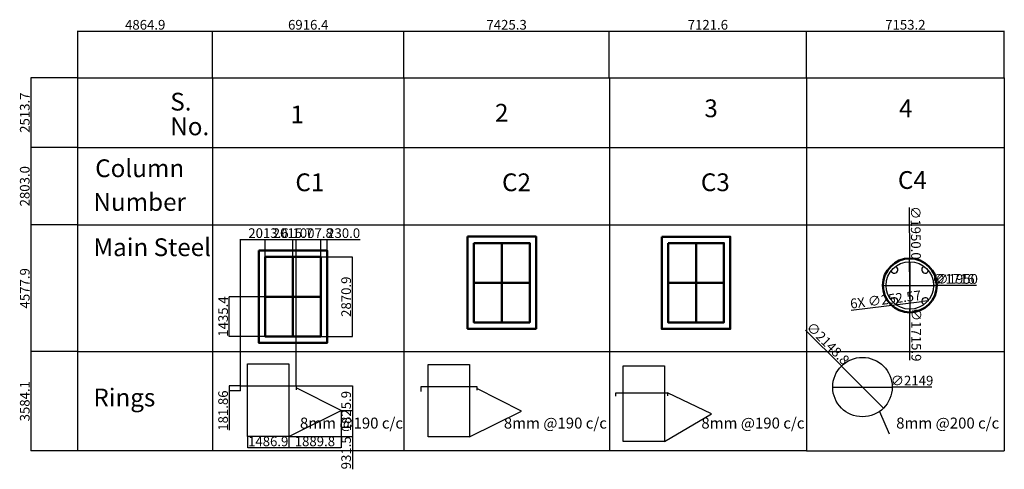
# Model space of a CAD drawing. Units: millimetres. Extents: x -2405 to 73447, y 417 to 55353.
# Tile 1 of 3: x 1710 to 37295, y 417 to 16669. Entities that reach past the tile are written whole.
import ezdxf

# ---------------------------------------------------------------- set-up
doc = ezdxf.new("R2010")
doc.units = ezdxf.units.MM
for name, color, linetype, lineweight in [('S-ANNO-DIMS', 2, 'Continuous', 18), ('S-ANNO-SCHD', 8, 'Continuous', 25), ('S-ANNO-TEXT', 7, 'Continuous', 25), ('S-COLS', 4, 'Continuous', 50), ('S-REIN', 1, 'Continuous', 25)]:
    doc.layers.add(name, color=color, linetype=linetype, lineweight=lineweight)
doc.styles.get("Standard").update_dxf_attribs({"font": 'arial.ttf'})
doc.dimstyles.new('ISO-25', dxfattribs={"dimtxt": 350, "dimasz": 2.5, "dimexe": 1.25, "dimexo": 0.625, "dimtad": 1, "dimdec": 0, "dimtxsty": 'Standard', "dimcen": 2.5, "dimadec": 0, "dimazin": 0, "dimtfac": 1, "dimtdec": 0, "dimtmove": 0, "dimatfit": 3, "dimfxl": 1, "dimarcsym": 0})

# ---------------------------------------------------------------- blocks, each defined once
blk = doc.blocks.new('COL-SECTION-RECT')
for p, q in [((1238, 230), (1238, 3101)), ((230, 1665), (2246, 1665))]:
    blk.add_line(p, q)
for points in [[(0, 3331), (2476, 3331), (2476, 0), (0, 0)], [(230, 3101), (2246, 3101), (2246, 230), (230, 230)]]:
    blk.add_lwpolyline(points, close=True)
blk = doc.blocks.new('RING-RECT')
for p, q in [((0, 1644), (0, 1826)), ((0, 1826), (2014, 1826)), ((2014, 1826), (2014, 1687)), ((3630, 932), (2014, 1756)), ((1740, 0), (3630, 932))]:
    blk.add_line(p, q)
blk.add_lwpolyline([(254, 2620), (1740, 2620), (1740, 0), (254, 0)], close=True)
blk = doc.blocks.new('*D37')
at = {"layer": 'Defpoints', "color": 0, "transparency": 16777216}
for p in [(31093, 3389), (33242, 3389)]:
    blk.add_point(p, dxfattribs=at)
at = {"layer": 'S-ANNO-DIMS', "color": 0, "lineweight": -2, "transparency": 16777216}
for p, q in [((31090, 3389), (31088, 3389)), ((31093, 3389), (33242, 3389)), ((34675, 3389), (33244, 3389))]:
    blk.add_line(p, q, dxfattribs=at)
at = {"layer": 'S-ANNO-DIMS', "color": 0, "transparency": 16777216}
for points in [[(31090, 3389), (31090, 3388), (31093, 3389)], [(33244, 3389), (33244, 3388), (33242, 3389)]]:
    blk.add_solid(points, dxfattribs=at)
at = {"layer": 'S-ANNO-DIMS', "color": 0, "transparency": 16777216, "insert": (33961, 3578), "char_height": 350, "attachment_point": 5, "rotation": 360}
blk.add_mtext('∅2149', dxfattribs=at)
blk = doc.blocks.new('*D38')
at = {"layer": 'Defpoints', "color": 0, "transparency": 16777216}
for p in [(32905, 7064), (34855, 7064)]:
    blk.add_point(p, dxfattribs=at)
at = {"layer": 'S-ANNO-DIMS', "color": 0, "lineweight": -2, "transparency": 16777216}
for p, q in [((32902, 7064), (32900, 7064)), ((32905, 7064), (34855, 7064)), ((36286, 7064), (34857, 7064))]:
    blk.add_line(p, q, dxfattribs=at)
at = {"layer": 'S-ANNO-DIMS', "color": 0, "transparency": 16777216}
for points in [[(32902, 7064), (32902, 7063), (32905, 7064)], [(34857, 7064), (34857, 7063), (34855, 7064)]]:
    blk.add_solid(points, dxfattribs=at)
at = {"layer": 'S-ANNO-DIMS', "color": 0, "transparency": 16777216, "insert": (35573, 7253), "char_height": 350, "attachment_point": 5, "rotation": 360}
blk.add_mtext('∅1950', dxfattribs=at)
blk = doc.blocks.new('*D39')
at = {"layer": 'Defpoints', "color": 0, "transparency": 16777216}
for p in [(33022, 7064), (34738, 7064)]:
    blk.add_point(p, dxfattribs=at)
at = {"layer": 'S-ANNO-DIMS', "color": 0, "lineweight": -2, "transparency": 16777216}
for p, q in [((33019, 7064), (33017, 7064)), ((33022, 7064), (34738, 7064)), ((36170, 7064), (34740, 7064))]:
    blk.add_line(p, q, dxfattribs=at)
at = {"layer": 'S-ANNO-DIMS', "color": 0, "transparency": 16777216}
for points in [[(33019, 7064), (33019, 7063), (33022, 7064)], [(34740, 7064), (34740, 7063), (34738, 7064)]]:
    blk.add_solid(points, dxfattribs=at)
at = {"layer": 'S-ANNO-DIMS', "color": 0, "transparency": 16777216, "insert": (35456, 7253), "char_height": 350, "attachment_point": 5, "rotation": 360}
blk.add_mtext('∅1716', dxfattribs=at)
blk = doc.blocks.new('*D63')
at = {"layer": 'Defpoints', "color": 0, "transparency": 16777216}
for p in [(12592, 8729), (10577, 8091), (12592, 8091)]:
    blk.add_point(p, dxfattribs=at)
at = {"layer": 'S-ANNO-DIMS', "color": 0, "lineweight": -2, "transparency": 16777216}
for p, q in [((10577, 8091), (10577, 8730)), ((10579, 8729), (12590, 8729)), ((12592, 8091), (12592, 8730))]:
    blk.add_line(p, q, dxfattribs=at)
at = {"layer": 'S-ANNO-DIMS', "color": 0, "transparency": 16777216}
for points in [[(10579, 8729), (10579, 8728), (10577, 8729)], [(12590, 8729), (12590, 8728), (12592, 8729)]]:
    blk.add_solid(points, dxfattribs=at)
at = {"layer": 'S-ANNO-DIMS', "color": 0, "transparency": 16777216, "insert": (11585, 8908), "char_height": 350, "attachment_point": 5}
blk.add_mtext('2015.7', dxfattribs=at)
blk = doc.blocks.new('*D64')
at = {"layer": 'Defpoints', "color": 0, "transparency": 16777216}
for p in [(12592, 8091), (13732, 8091), (12592, 5220)]:
    blk.add_point(p, dxfattribs=at)
at = {"layer": 'S-ANNO-DIMS', "color": 0, "lineweight": -2, "transparency": 16777216}
for p, q in [((12593, 8091), (13733, 8091)), ((13732, 5222), (13732, 8088)), ((12593, 5220), (13733, 5220))]:
    blk.add_line(p, q, dxfattribs=at)
at = {"layer": 'S-ANNO-DIMS', "color": 0, "transparency": 16777216}
for points in [[(13732, 8088), (13732, 8088), (13732, 8091)], [(13732, 5222), (13732, 5222), (13732, 5220)]]:
    blk.add_solid(points, dxfattribs=at)
at = {"layer": 'S-ANNO-DIMS', "color": 0, "transparency": 16777216, "insert": (13553, 6655), "char_height": 350, "attachment_point": 5, "rotation": 90}
blk.add_mtext('2870.9', dxfattribs=at)
blk = doc.blocks.new('*D65')
at = {"layer": 'Defpoints', "color": 0, "transparency": 16777216}
for p in [(12822, 8729), (12822, 8321), (12592, 8091)]:
    blk.add_point(p, dxfattribs=at)
at = {"layer": 'S-ANNO-DIMS', "color": 0, "lineweight": -2, "transparency": 16777216}
for p, q in [((12592, 8091), (12592, 8730)), ((12595, 8729), (12820, 8729)), ((12822, 8321), (12822, 8730)), ((12822, 8729), (14012, 8729))]:
    blk.add_line(p, q, dxfattribs=at)
at = {"layer": 'S-ANNO-DIMS', "color": 0, "transparency": 16777216}
for points in [[(12595, 8729), (12595, 8728), (12592, 8729)], [(12820, 8729), (12820, 8728), (12822, 8729)]]:
    blk.add_solid(points, dxfattribs=at)
at = {"layer": 'S-ANNO-DIMS', "color": 0, "transparency": 16777216, "insert": (13418, 8908), "char_height": 350, "attachment_point": 5}
blk.add_mtext('230.0', dxfattribs=at)
blk = doc.blocks.new('*D66')
at = {"layer": 'Defpoints', "color": 0, "transparency": 16777216}
for p in [(11585, 8729), (10577, 8091), (11585, 8091)]:
    blk.add_point(p, dxfattribs=at)
at = {"layer": 'S-ANNO-DIMS', "color": 0, "lineweight": -2, "transparency": 16777216}
for p, q in [((10577, 8091), (10577, 8730)), ((10579, 8729), (11582, 8729)), ((11585, 8091), (11585, 8730)), ((11585, 8729), (13009, 8729))]:
    blk.add_line(p, q, dxfattribs=at)
at = {"layer": 'S-ANNO-DIMS', "color": 0, "transparency": 16777216}
for points in [[(10579, 8729), (10579, 8728), (10577, 8729)], [(11582, 8729), (11582, 8728), (11585, 8729)]]:
    blk.add_solid(points, dxfattribs=at)
at = {"layer": 'S-ANNO-DIMS', "color": 0, "transparency": 16777216, "insert": (12298, 8908), "char_height": 350, "attachment_point": 5}
blk.add_mtext('1007.8', dxfattribs=at)
blk = doc.blocks.new('*D67')
at = {"layer": 'Defpoints', "color": 0, "transparency": 16777216}
for p in [(9286, 6655), (10577, 6655), (10577, 5220)]:
    blk.add_point(p, dxfattribs=at)
at = {"layer": 'S-ANNO-DIMS', "color": 0, "lineweight": -2, "transparency": 16777216}
for p, q in [((10576, 6655), (9285, 6655)), ((9286, 5222), (9286, 6653)), ((10576, 5220), (9285, 5220))]:
    blk.add_line(p, q, dxfattribs=at)
at = {"layer": 'S-ANNO-DIMS', "color": 0, "transparency": 16777216}
for points in [[(9286, 6653), (9286, 6653), (9286, 6655)], [(9286, 5222), (9286, 5222), (9286, 5220)]]:
    blk.add_solid(points, dxfattribs=at)
at = {"layer": 'S-ANNO-DIMS', "color": 0, "transparency": 16777216, "insert": (9107, 5938), "char_height": 350, "attachment_point": 5, "rotation": 90}
blk.add_mtext('1435.4', dxfattribs=at)
blk = doc.blocks.new('*D68')
at = {"layer": 'Defpoints', "color": 0, "transparency": 16777216}
for p in [(9947, 1608), (11434, 1608), (11434, 1200)]:
    blk.add_point(p, dxfattribs=at)
at = {"layer": 'S-ANNO-DIMS', "color": 0, "lineweight": -2, "transparency": 16777216}
for p, q in [((9947, 1608), (9947, 1199)), ((11434, 1608), (11434, 1199)), ((9950, 1200), (11432, 1200))]:
    blk.add_line(p, q, dxfattribs=at)
at = {"layer": 'S-ANNO-DIMS', "color": 0, "transparency": 16777216}
for points in [[(9950, 1201), (9950, 1200), (9947, 1200)], [(11432, 1201), (11432, 1200), (11434, 1200)]]:
    blk.add_solid(points, dxfattribs=at)
at = {"layer": 'S-ANNO-DIMS', "color": 0, "transparency": 16777216, "insert": (10691, 1380), "char_height": 350, "attachment_point": 5}
blk.add_mtext('1486.9', dxfattribs=at)
blk = doc.blocks.new('*D69')
at = {"layer": 'Defpoints', "color": 0, "transparency": 16777216}
for p in [(11707, 8729), (9694, 3434), (11707, 3434)]:
    blk.add_point(p, dxfattribs=at)
at = {"layer": 'S-ANNO-DIMS', "color": 0, "lineweight": -2, "transparency": 16777216}
for p, q in [((9694, 3435), (9694, 8730)), ((9696, 8729), (11705, 8729)), ((11707, 3435), (11707, 8730))]:
    blk.add_line(p, q, dxfattribs=at)
at = {"layer": 'S-ANNO-DIMS', "color": 0, "transparency": 16777216}
for points in [[(9696, 8729), (9696, 8728), (9694, 8729)], [(11705, 8729), (11705, 8728), (11707, 8729)]]:
    blk.add_solid(points, dxfattribs=at)
at = {"layer": 'S-ANNO-DIMS', "color": 0, "transparency": 16777216, "insert": (10701, 8908), "char_height": 350, "attachment_point": 5}
blk.add_mtext('2013.6', dxfattribs=at)
blk = doc.blocks.new('*D70')
at = {"layer": 'Defpoints', "color": 0, "transparency": 16777216}
for p in [(9286, 3252), (9694, 3434), (9694, 3252)]:
    blk.add_point(p, dxfattribs=at)
at = {"layer": 'S-ANNO-DIMS', "color": 0, "lineweight": -2, "transparency": 16777216}
for p, q in [((9693, 3434), (9285, 3434)), ((9693, 3252), (9285, 3252)), ((9286, 3432), (9286, 3255)), ((9286, 3252), (9286, 1829))]:
    blk.add_line(p, q, dxfattribs=at)
at = {"layer": 'S-ANNO-DIMS', "color": 0, "transparency": 16777216}
for points in [[(9286, 3432), (9286, 3432), (9286, 3434)], [(9286, 3255), (9286, 3255), (9286, 3252)]]:
    blk.add_solid(points, dxfattribs=at)
at = {"layer": 'S-ANNO-DIMS', "color": 0, "transparency": 16777216, "insert": (9107, 2539), "char_height": 350, "attachment_point": 5, "rotation": 90}
blk.add_mtext('181.86', dxfattribs=at)
blk = doc.blocks.new('*D71')
at = {"layer": 'Defpoints', "color": 0, "transparency": 16777216}
for p in [(11707, 3434), (11434, 1608), (13732, 1608)]:
    blk.add_point(p, dxfattribs=at)
at = {"layer": 'S-ANNO-DIMS', "color": 0, "lineweight": -2, "transparency": 16777216}
for p, q in [((11708, 3434), (13733, 3434)), ((13732, 3432), (13732, 1611)), ((11435, 1608), (13733, 1608))]:
    blk.add_line(p, q, dxfattribs=at)
at = {"layer": 'S-ANNO-DIMS', "color": 0, "transparency": 16777216}
for points in [[(13732, 3432), (13732, 3432), (13732, 3434)], [(13732, 1611), (13732, 1611), (13732, 1608)]]:
    blk.add_solid(points, dxfattribs=at)
at = {"layer": 'S-ANNO-DIMS', "color": 0, "transparency": 16777216, "insert": (13553, 2521), "char_height": 350, "attachment_point": 5, "rotation": 90}
blk.add_mtext('1825.9', dxfattribs=at)
blk = doc.blocks.new('*D72')
at = {"layer": 'Defpoints', "color": 0, "transparency": 16777216}
for p in [(13324, 2540), (11434, 1608), (13324, 1200)]:
    blk.add_point(p, dxfattribs=at)
at = {"layer": 'S-ANNO-DIMS', "color": 0, "lineweight": -2, "transparency": 16777216}
for p, q in [((13324, 2539), (13324, 1199)), ((11434, 1608), (11434, 1199)), ((11437, 1200), (13322, 1200))]:
    blk.add_line(p, q, dxfattribs=at)
at = {"layer": 'S-ANNO-DIMS', "color": 0, "transparency": 16777216}
for points in [[(11437, 1201), (11437, 1200), (11434, 1200)], [(13322, 1201), (13322, 1200), (13324, 1200)]]:
    blk.add_solid(points, dxfattribs=at)
at = {"layer": 'S-ANNO-DIMS', "color": 0, "transparency": 16777216, "insert": (12379, 1380), "char_height": 350, "attachment_point": 5}
blk.add_mtext('1889.8', dxfattribs=at)
blk = doc.blocks.new('*D73')
at = {"layer": 'Defpoints', "color": 0, "transparency": 16777216}
for p in [(13324, 2540), (11434, 1608), (13732, 1608)]:
    blk.add_point(p, dxfattribs=at)
at = {"layer": 'S-ANNO-DIMS', "color": 0, "lineweight": -2, "transparency": 16777216}
for p, q in [((13325, 2540), (13733, 2540)), ((13732, 2537), (13732, 1611)), ((11435, 1608), (13733, 1608)), ((13732, 1608), (13732, 421))]:
    blk.add_line(p, q, dxfattribs=at)
at = {"layer": 'S-ANNO-DIMS', "color": 0, "transparency": 16777216}
for points in [[(13732, 2537), (13732, 2537), (13732, 2540)], [(13732, 1611), (13732, 1611), (13732, 1608)]]:
    blk.add_solid(points, dxfattribs=at)
at = {"layer": 'S-ANNO-DIMS', "color": 0, "transparency": 16777216, "insert": (13553, 1013), "char_height": 350, "attachment_point": 5, "rotation": 90}
blk.add_mtext('931.5', dxfattribs=at)
blk = doc.blocks.new('*D74')
at = {"layer": 'Defpoints', "color": 0, "transparency": 16777216}
for p in [(8679, 16259), (3814, 14564), (8679, 14564)]:
    blk.add_point(p, dxfattribs=at)
at = {"layer": 'S-ANNO-DIMS', "color": 0, "lineweight": -2, "transparency": 16777216}
for p, q in [((3814, 14565), (3814, 16261)), ((3816, 16259), (8676, 16259)), ((8679, 14565), (8679, 16261))]:
    blk.add_line(p, q, dxfattribs=at)
at = {"layer": 'S-ANNO-DIMS', "color": 0, "transparency": 16777216}
for points in [[(3816, 16260), (3816, 16259), (3814, 16259)], [(8676, 16260), (8676, 16259), (8679, 16259)]]:
    blk.add_solid(points, dxfattribs=at)
at = {"layer": 'S-ANNO-DIMS', "color": 0, "transparency": 16777216, "insert": (6246, 16439), "char_height": 350, "attachment_point": 5}
blk.add_mtext('4864.9', dxfattribs=at)
blk = doc.blocks.new('*D75')
at = {"layer": 'Defpoints', "color": 0, "transparency": 16777216}
for p in [(15595, 16259), (8679, 14564), (15595, 14564)]:
    blk.add_point(p, dxfattribs=at)
at = {"layer": 'S-ANNO-DIMS', "color": 0, "lineweight": -2, "transparency": 16777216}
for p, q in [((8679, 14565), (8679, 16261)), ((8681, 16259), (15593, 16259)), ((15595, 14565), (15595, 16261))]:
    blk.add_line(p, q, dxfattribs=at)
at = {"layer": 'S-ANNO-DIMS', "color": 0, "transparency": 16777216}
for points in [[(8681, 16260), (8681, 16259), (8679, 16259)], [(15593, 16260), (15593, 16259), (15595, 16259)]]:
    blk.add_solid(points, dxfattribs=at)
at = {"layer": 'S-ANNO-DIMS', "color": 0, "transparency": 16777216, "insert": (12137, 16439), "char_height": 350, "attachment_point": 5}
blk.add_mtext('6916.4', dxfattribs=at)
blk = doc.blocks.new('*D76')
at = {"layer": 'Defpoints', "color": 0, "transparency": 16777216}
for p in [(23020, 16259), (15595, 14564), (23020, 14564)]:
    blk.add_point(p, dxfattribs=at)
at = {"layer": 'S-ANNO-DIMS', "color": 0, "lineweight": -2, "transparency": 16777216}
for p, q in [((15595, 14565), (15595, 16261)), ((15598, 16259), (23018, 16259)), ((23020, 14565), (23020, 16261))]:
    blk.add_line(p, q, dxfattribs=at)
at = {"layer": 'S-ANNO-DIMS', "color": 0, "transparency": 16777216}
for points in [[(15598, 16260), (15598, 16259), (15595, 16259)], [(23018, 16260), (23018, 16259), (23020, 16259)]]:
    blk.add_solid(points, dxfattribs=at)
at = {"layer": 'S-ANNO-DIMS', "color": 0, "transparency": 16777216, "insert": (19308, 16439), "char_height": 350, "attachment_point": 5}
blk.add_mtext('7425.3', dxfattribs=at)
blk = doc.blocks.new('*D77')
at = {"layer": 'Defpoints', "color": 0, "transparency": 16777216}
for p in [(30142, 16259), (23020, 14564), (30142, 14564)]:
    blk.add_point(p, dxfattribs=at)
at = {"layer": 'S-ANNO-DIMS', "color": 0, "lineweight": -2, "transparency": 16777216}
for p, q in [((23020, 14565), (23020, 16261)), ((23023, 16259), (30139, 16259)), ((30142, 14565), (30142, 16261))]:
    blk.add_line(p, q, dxfattribs=at)
at = {"layer": 'S-ANNO-DIMS', "color": 0, "transparency": 16777216}
for points in [[(23023, 16260), (23023, 16259), (23020, 16259)], [(30139, 16260), (30139, 16259), (30142, 16259)]]:
    blk.add_solid(points, dxfattribs=at)
at = {"layer": 'S-ANNO-DIMS', "color": 0, "transparency": 16777216, "insert": (26581, 16439), "char_height": 350, "attachment_point": 5}
blk.add_mtext('7121.6', dxfattribs=at)
blk = doc.blocks.new('*D78')
at = {"layer": 'Defpoints', "color": 0, "transparency": 16777216}
for p in [(37295, 16259), (30142, 14564), (37295, 14564)]:
    blk.add_point(p, dxfattribs=at)
at = {"layer": 'S-ANNO-DIMS', "color": 0, "lineweight": -2, "transparency": 16777216}
for p, q in [((30142, 14565), (30142, 16261)), ((30144, 16259), (37293, 16259)), ((37295, 14565), (37295, 16261))]:
    blk.add_line(p, q, dxfattribs=at)
at = {"layer": 'S-ANNO-DIMS', "color": 0, "transparency": 16777216}
for points in [[(30144, 16260), (30144, 16259), (30142, 16259)], [(37293, 16260), (37293, 16259), (37295, 16259)]]:
    blk.add_solid(points, dxfattribs=at)
at = {"layer": 'S-ANNO-DIMS', "color": 0, "transparency": 16777216, "insert": (33719, 16439), "char_height": 350, "attachment_point": 5}
blk.add_mtext('7153.2', dxfattribs=at)
blk = doc.blocks.new('*D79')
at = {"layer": 'Defpoints', "color": 0, "transparency": 16777216}
for p in [(2119, 4670), (3814, 4670), (3814, 1086)]:
    blk.add_point(p, dxfattribs=at)
at = {"layer": 'S-ANNO-DIMS', "color": 0, "lineweight": -2, "transparency": 16777216}
for p, q in [((3813, 4670), (2118, 4670)), ((2119, 1088), (2119, 4667)), ((3813, 1086), (2118, 1086))]:
    blk.add_line(p, q, dxfattribs=at)
at = {"layer": 'S-ANNO-DIMS', "color": 0, "transparency": 16777216}
for points in [[(2118, 4667), (2119, 4667), (2119, 4670)], [(2118, 1088), (2119, 1088), (2119, 1086)]]:
    blk.add_solid(points, dxfattribs=at)
at = {"layer": 'S-ANNO-DIMS', "color": 0, "transparency": 16777216, "insert": (1939, 2878), "char_height": 350, "attachment_point": 5, "rotation": 90}
blk.add_mtext('3584.1', dxfattribs=at)
blk = doc.blocks.new('*D80')
at = {"layer": 'Defpoints', "color": 0, "transparency": 16777216}
for p in [(2119, 9248), (3814, 9248), (3814, 4670)]:
    blk.add_point(p, dxfattribs=at)
at = {"layer": 'S-ANNO-DIMS', "color": 0, "lineweight": -2, "transparency": 16777216}
for p, q in [((3813, 9248), (2118, 9248)), ((2119, 4672), (2119, 9245)), ((3813, 4670), (2118, 4670))]:
    blk.add_line(p, q, dxfattribs=at)
at = {"layer": 'S-ANNO-DIMS', "color": 0, "transparency": 16777216}
for points in [[(2118, 9245), (2119, 9245), (2119, 9248)], [(2118, 4672), (2119, 4672), (2119, 4670)]]:
    blk.add_solid(points, dxfattribs=at)
at = {"layer": 'S-ANNO-DIMS', "color": 0, "transparency": 16777216, "insert": (1939, 6959), "char_height": 350, "attachment_point": 5, "rotation": 90}
blk.add_mtext('4577.9', dxfattribs=at)
blk = doc.blocks.new('*D81')
at = {"layer": 'Defpoints', "color": 0, "transparency": 16777216}
for p in [(2119, 12051), (3814, 12051), (3814, 9248)]:
    blk.add_point(p, dxfattribs=at)
at = {"layer": 'S-ANNO-DIMS', "color": 0, "lineweight": -2, "transparency": 16777216}
for p, q in [((3813, 12051), (2118, 12051)), ((2119, 9250), (2119, 12048)), ((3813, 9248), (2118, 9248))]:
    blk.add_line(p, q, dxfattribs=at)
at = {"layer": 'S-ANNO-DIMS', "color": 0, "transparency": 16777216}
for points in [[(2118, 12048), (2119, 12048), (2119, 12051)], [(2118, 9250), (2119, 9250), (2119, 9248)]]:
    blk.add_solid(points, dxfattribs=at)
at = {"layer": 'S-ANNO-DIMS', "color": 0, "transparency": 16777216, "insert": (1939, 10649), "char_height": 350, "attachment_point": 5, "rotation": 90}
blk.add_mtext('2803.0', dxfattribs=at)
blk = doc.blocks.new('*D82')
at = {"layer": 'Defpoints', "color": 0, "transparency": 16777216}
for p in [(2119, 14564), (3814, 14564), (3814, 12051)]:
    blk.add_point(p, dxfattribs=at)
at = {"layer": 'S-ANNO-DIMS', "color": 0, "lineweight": -2, "transparency": 16777216}
for p, q in [((3813, 14564), (2118, 14564)), ((2119, 12053), (2119, 14562)), ((3813, 12051), (2118, 12051))]:
    blk.add_line(p, q, dxfattribs=at)
at = {"layer": 'S-ANNO-DIMS', "color": 0, "transparency": 16777216}
for points in [[(2118, 14562), (2119, 14562), (2119, 14564)], [(2118, 12053), (2119, 12053), (2119, 12051)]]:
    blk.add_solid(points, dxfattribs=at)
at = {"layer": 'S-ANNO-DIMS', "color": 0, "transparency": 16777216, "insert": (1939, 13308), "char_height": 350, "attachment_point": 5, "rotation": 90}
blk.add_mtext('2513.7', dxfattribs=at)
blk = doc.blocks.new('*D83')
at = {"layer": 'Defpoints', "color": 0, "transparency": 16777216}
for p in [(31408, 4149), (32927, 2628)]:
    blk.add_point(p, dxfattribs=at)
at = {"layer": 'S-ANNO-DIMS', "color": 0, "lineweight": -2, "transparency": 16777216}
for p, q in [((30107, 5451), (31406, 4151)), ((32927, 2628), (31408, 4149)), ((32928, 2627), (32930, 2625))]:
    blk.add_line(p, q, dxfattribs=at)
at = {"layer": 'S-ANNO-DIMS', "color": 0, "transparency": 16777216}
for points in [[(31407, 4151), (31406, 4150), (31408, 4149)], [(32929, 2627), (32928, 2626), (32927, 2628)]]:
    blk.add_solid(points, dxfattribs=at)
at = {"layer": 'S-ANNO-DIMS', "color": 0, "transparency": 16777216, "insert": (30890, 4935), "char_height": 350, "attachment_point": 5, "rotation": 314.9629}
blk.add_mtext('∅2148.8', dxfattribs=at)
blk = doc.blocks.new('*D84')
at = {"layer": 'Defpoints', "color": 0, "transparency": 16777216}
for p in [(33870, 8039), (33890, 6089)]:
    blk.add_point(p, dxfattribs=at)
at = {"layer": 'S-ANNO-DIMS', "color": 0, "lineweight": -2, "transparency": 16777216}
for p, q in [((33851, 9877), (33870, 8041)), ((33890, 6089), (33870, 8039)), ((33890, 6086), (33890, 6084))]:
    blk.add_line(p, q, dxfattribs=at)
at = {"layer": 'S-ANNO-DIMS', "color": 0, "transparency": 16777216}
for points in [[(33870, 8041), (33870, 8041), (33870, 8039)], [(33890, 6086), (33889, 6086), (33890, 6089)]]:
    blk.add_solid(points, dxfattribs=at)
at = {"layer": 'S-ANNO-DIMS', "color": 0, "transparency": 16777216, "insert": (34050, 8962), "char_height": 350, "attachment_point": 5, "rotation": 270.5813}
blk.add_mtext('∅1950.0', dxfattribs=at)
blk = doc.blocks.new('*D85')
at = {"layer": 'Defpoints', "color": 0, "transparency": 16777216}
for p in [(33880, 7922), (33880, 6206)]:
    blk.add_point(p, dxfattribs=at)
at = {"layer": 'S-ANNO-DIMS', "color": 0, "lineweight": -2, "transparency": 16777216}
for p, q in [((33880, 7924), (33880, 7927)), ((33880, 7922), (33880, 6206)), ((33880, 4365), (33880, 6203))]:
    blk.add_line(p, q, dxfattribs=at)
at = {"layer": 'S-ANNO-DIMS', "color": 0, "transparency": 16777216}
for points in [[(33880, 7924), (33879, 7924), (33880, 7922)], [(33880, 6203), (33880, 6203), (33880, 6206)]]:
    blk.add_solid(points, dxfattribs=at)
at = {"layer": 'S-ANNO-DIMS', "color": 0, "transparency": 16777216, "insert": (34069, 5283), "char_height": 350, "attachment_point": 5, "rotation": 270.0069}
blk.add_mtext('∅1715.9', dxfattribs=at)
blk = doc.blocks.new('*D86')
at = {"layer": 'Defpoints', "color": 0, "transparency": 16777216}
for p in [(34314, 6479), (34565, 6510)]:
    blk.add_point(p, dxfattribs=at)
at = {"layer": 'S-ANNO-DIMS', "color": 0, "lineweight": -2, "transparency": 16777216}
for p, q in [((31758, 6166), (34312, 6479)), ((34565, 6510), (34314, 6479)), ((34567, 6510), (34570, 6511))]:
    blk.add_line(p, q, dxfattribs=at)
at = {"layer": 'S-ANNO-DIMS', "color": 0, "transparency": 16777216}
for points in [[(34312, 6480), (34312, 6479), (34314, 6479)], [(34567, 6511), (34567, 6510), (34565, 6510)]]:
    blk.add_solid(points, dxfattribs=at)
at = {"layer": 'S-ANNO-DIMS', "color": 0, "transparency": 16777216, "insert": (33011, 6510), "char_height": 350, "attachment_point": 5, "rotation": 6.983}
blk.add_mtext('6X ∅252.57', dxfattribs=at)

msp = doc.modelspace()

# ---------------------------------------------------------------- linework, layer by layer
at = {"layer": 'S-ANNO-SCHD'}
for p, q in [((8678.624, 14564.391), (8678.624, 1085.686)), ((15595.007, 14564.391), (15595.007, 1085.686)), ((23020.311, 14564.391), (23020.311, 1085.686)), ((30141.945, 14564.391), (37295.175, 14564.391)), ((37295.175, 14564.391), (37295.175, 1085.686)), ((3813.765, 12050.714), (30141.945, 12050.714)), ((30141.945, 12050.714), (37295.175, 12050.714)), ((3813.765, 9247.67), (30141.945, 9247.67)), ((30141.945, 9247.67), (37295.175, 9247.67)), ((3813.765, 4669.757), (30141.945, 4669.757)), ((30141.945, 4669.757), (37295.175, 4669.757)), ((30141.945, 1085.686), (37295.175, 1085.686))]:
    msp.add_line(p, q, dxfattribs=at)
msp.add_lwpolyline([(3813.765, 14564.391), (30141.945, 14564.391), (30141.945, 1085.686), (3813.765, 1085.686)], close=True, dxfattribs=at)
at = {"layer": 'S-COLS'}
msp.add_circle((33879.896, 7063.577), 974.982, dxfattribs=at)
at = {"layer": 'S-REIN'}
for p, q in [((33879.896, 7921.52), (33879.896, 6205.635)), ((33021.954, 7063.577), (34737.839, 7063.577)), ((23251.426, 3057.547), (23251.426, 3176.771)), ((23251.426, 3176.771), (25118.601, 3176.771)), ((25118.601, 3176.771), (25118.601, 3068.643)), ((26713.261, 2425.091), (25118.601, 3176.771)), ((32788.957, 2512.323), (33135.891, 1695.25)), ((25011.082, 1419.692), (26713.261, 2425.091))]:
    msp.add_line(p, q, dxfattribs=at)
msp.add_lwpolyline([(23522.542, 4159.482), (25011.082, 4159.482), (25011.082, 1419.692), (23522.542, 1419.692)], close=True, dxfattribs=at)
for centre, radius in [((33879.896, 7063.577), 857.943), ((32167.361, 3388.654), 1074.402)]:
    msp.add_circle(centre, radius, dxfattribs=at)
for centre, start, end in [((33320.276, 7632.366), 200.0821557, 68.9867935), ((34439.517, 7632.366), 111.0132065, 339.9178443), ((33320.276, 6494.788), 291.0132065, 159.9178443), ((34439.517, 6494.788), 20.0821557, 248.9867935)]:
    msp.add_arc(centre, 126.284, start, end, dxfattribs=at)

# ---------------------------------------------------------------- block references
at = {"layer": 'S-COLS'}
for p in [(17896.73, 5495.397), (24916.373, 5494.104), (10346.781, 4989.9)]:
    msp.add_blockref('COL-SECTION-RECT', p, dxfattribs=at)
at = {"layer": 'S-REIN'}
for p in [(9693.868, 1608.18), (16220.79, 1586.288)]:
    msp.add_blockref('RING-RECT', p, dxfattribs=at)

# ---------------------------------------------------------------- texts
at = {"layer": 'S-ANNO-TEXT'}
for s, height, p in [('S.', 642.3597, (7151.838, 13384.262)), ('1', 642.36, (11498.701, 12921.972)), ('2', 642.36, (18887.719, 12983.301)), ('3', 642.36, (26454.48, 13144.098)), ('4', 642.36, (33490.288, 13144.098)), ('No.', 642.3597, (7151.838, 12491.225)), ('Column', 642.3597, (4437.932, 10977.642)), ('C1', 642.3597, (11673.595, 10469.528)), ('C2', 642.3597, (19141.63, 10469.528)), ('C3', 642.3597, (26328.181, 10471.367)), ('C4', 642.3597, (33450.482, 10552.433)), ('Number', 642.3597, (4373.727, 9759.251)), ('Main Steel', 642.3597, (4373.727, 8123.346)), ('Rings', 642.3597, (4373.727, 2691.81)), ('8mm @190 c/c', 396.94498, (11838.205, 1889.496)), ('8mm @190 c/c', 396.94498, (19208.198, 1889.496)), ('8mm @190 c/c', 396.94498, (26346.879, 1889.496)), ('8mm @200 c/c', 396.94498, (33387.063, 1889.496))]:
    msp.add_text(s, height=height, dxfattribs=at).set_placement(p)

# ---------------------------------------------------------------- dimensions: what is measured, and where the dimension line sits
at = {"layer": 'S-ANNO-DIMS'}
for base, p1, p2, picture, middle in [((8678.624, 16259.391), (3813.765, 14564.391), (8678.624, 14564.391), '*D74', (6246.195, 16438.716)), ((15595.007, 16259.391), (8678.624, 14564.391), (15595.007, 14564.391), '*D75', (12136.816, 16438.716)), ((23020.311, 16259.391), (15595.007, 14564.391), (23020.311, 14564.391), '*D76', (19307.659, 16438.836)), ((30141.945, 16259.391), (23020.311, 14564.391), (30141.945, 14564.391), '*D77', (26581.128, 16438.716)), ((37295.175, 16259.391), (30141.945, 14564.391), (37295.175, 14564.391), '*D78', (33718.56, 16438.836)), ((11707.493, 8728.615), (9693.868, 3434.097), (11707.493, 3434.097), '*D69', (10700.681, 8908.06)), ((12592.433, 8728.615), (10576.781, 8090.765), (12592.433, 8090.765), '*D63', (11584.607, 8907.941)), ((11584.607, 8728.615), (10576.781, 8090.765), (11584.607, 8090.765), '*D66', (12298.117, 8907.941)), ((12822.433, 8728.615), (12592.433, 8090.765), (12822.433, 8320.765), '*D65', (13418.481, 8908.06)), ((13324.153, 1200.33), (11434.365, 1608.18), (13324.153, 2539.682), '*D72', (12379.259, 1379.655)), ((11434.365, 1200.33), (9947.463, 1608.18), (11434.365, 1608.18), '*D68', (10690.914, 1379.655))]:
    dim = msp.add_linear_dim(base=base, p1=p1, p2=p2, dimstyle='ISO-25', override={"dimdec": 1, "dimlfac": 1, "dimrnd": 0, "dimzin": 0, "dimdsep": 46, "dimlunit": 2}, dxfattribs=at)
    dim.commit()
    dim.dimension.update_dxf_attribs({"geometry": picture, "text_midpoint": middle})
for base, p1, p2, override, picture, middle in [((2118.765, 14564.391), (3813.765, 12050.714), (3813.765, 14564.391), {"dimdec": 1, "dimlfac": 1, "dimrnd": 0, "dimzin": 0, "dimdsep": 46, "dimlunit": 2}, '*D82', (1939.321, 13307.552)), ((2118.765, 12050.714), (3813.765, 9247.67), (3813.765, 12050.714), {"dimdec": 1, "dimlfac": 1, "dimrnd": 0, "dimzin": 0, "dimdsep": 46, "dimlunit": 2}, '*D81', (1939.321, 10649.192)), ((2118.765, 9247.67), (3813.765, 4669.757), (3813.765, 9247.67), {"dimdec": 1, "dimlfac": 1, "dimrnd": 0, "dimzin": 0, "dimdsep": 46, "dimlunit": 2}, '*D80', (1939.44, 6958.713)), ((13732.003, 8090.765), (12592.433, 5219.9), (12592.433, 8090.765), {"dimdec": 1, "dimlfac": 1, "dimrnd": 0, "dimzin": 0, "dimdsep": 46, "dimlunit": 2}, '*D64', (13552.677, 6655.333)), ((9286.018, 6655.333), (10576.781, 5219.9), (10576.781, 6655.333), {"dimdec": 1, "dimlfac": 1, "dimrnd": 0, "dimzin": 0, "dimdsep": 46, "dimlunit": 2}, '*D67', (9106.573, 5937.616)), ((2118.765, 4669.757), (3813.765, 1085.686), (3813.765, 4669.757), {"dimdec": 1, "dimlfac": 1, "dimrnd": 0, "dimzin": 0, "dimdsep": 46, "dimlunit": 2}, '*D79', (1939.321, 2877.722)), ((9286.018, 3252.238), (9693.868, 3434.097), (9693.868, 3252.238), {"dimdec": 2, "dimlfac": 1, "dimrnd": 0, "dimzin": 0, "dimdsep": 46, "dimlunit": 2}, '*D70', (9106.693, 2539.205)), ((13732.003, 1608.18), (11707.493, 3434.097), (11434.365, 1608.18), {"dimdec": 1, "dimlfac": 1, "dimrnd": 0, "dimzin": 0, "dimdsep": 46, "dimlunit": 2}, '*D71', (13552.677, 2521.138)), ((13732.003, 1608.18), (13324.153, 2539.682), (11434.365, 1608.18), {"dimdec": 1, "dimlfac": 1, "dimrnd": 0, "dimzin": 0, "dimdsep": 46, "dimlunit": 2}, '*D73', (13552.558, 1013.206))]:
    dim = msp.add_linear_dim(base=base, p1=p1, p2=p2, angle=90, dimstyle='ISO-25', override=override, dxfattribs=at)
    dim.commit()
    dim.dimension.update_dxf_attribs({"geometry": picture, "text_midpoint": middle})
for p1, p2, override, picture, middle in [((33889.787, 6088.645), (33870.005, 8038.509), {"dimdec": 1, "dimlfac": 1, "dimrnd": 0, "dimzin": 0, "dimdsep": 46, "dimlunit": 2}, '*D84', (33860.652, 8960.39)), ((32904.914, 7063.577), (34854.879, 7063.577), {"dimdec": 0, "dimlfac": 1, "dimrnd": 0, "dimzin": 0, "dimdsep": 46, "dimlunit": 2}, '*D38', (35572.918, 7063.577)), ((32926.585, 2628.445), (31408.137, 4148.863), {"dimdec": 1, "dimlfac": 1, "dimrnd": 0, "dimzin": 0, "dimdsep": 46, "dimlunit": 2}, '*D83', (30755.983, 4801.863)), ((31092.959, 3388.655), (33241.763, 3388.654), {"dimdec": 0, "dimlfac": 1, "dimrnd": 0, "dimzin": 0, "dimdsep": 46, "dimlunit": 2}, '*D37', (33960.758, 3388.654))]:
    dim = msp.add_diameter_dim_2p(p1=p1, p2=p2, dimstyle='ISO-25', override=override, dxfattribs=at)
    dim.commit()
    dim.dimension.update_dxf_attribs({"geometry": picture, "text_midpoint": middle})
for p1, p2, override, picture, middle in [((33879.792, 7921.52), (33880, 6205.635), {"dimdec": 1, "dimlfac": 1, "dimrnd": 0, "dimzin": 0, "dimdsep": 46, "dimlunit": 2}, '*D85', (33880.112, 5282.752)), ((33021.954, 7063.577), (34737.839, 7063.577), {"dimdec": 0, "dimlfac": 1, "dimrnd": 0, "dimzin": 0, "dimdsep": 46, "dimlunit": 2}, '*D39', (35456.356, 7063.577))]:
    dim = msp.add_diameter_dim_2p(p1=p1, p2=p2, dimstyle='ISO-25', override=override, dxfattribs=at)
    dim.commit()
    dim.dimension.update_dxf_attribs({"geometry": picture, "text_midpoint": middle, "dimtype": 163})
dim = msp.add_diameter_dim_2p(p1=(34564.864, 6510.141), p2=(34314.169, 6479.435), text='6X <>', dimstyle='ISO-25', override={"dimdec": 2, "dimlfac": 1, "dimrnd": 0, "dimzin": 0, "dimdsep": 46, "dimlunit": 2}, dxfattribs=at)
dim.commit()
dim.dimension.update_dxf_attribs({"geometry": '*D86', "text_midpoint": (33033.548, 6322.58), "dimtype": 163})

doc.saveas('drawing.dxf')
